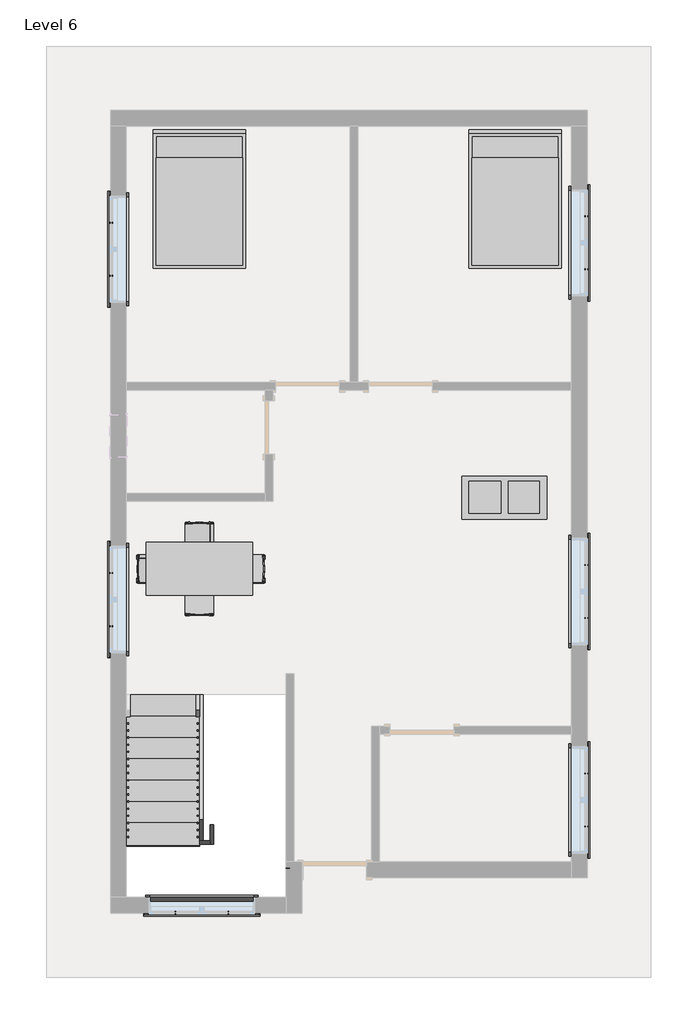
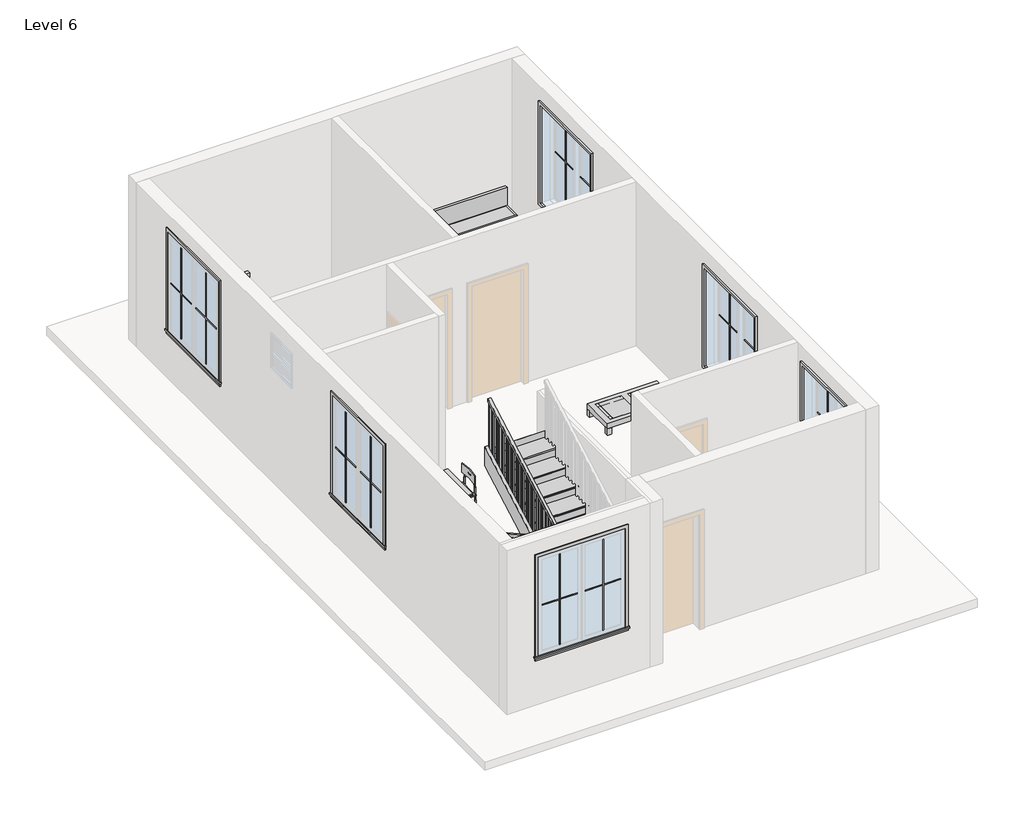
# One storey, part 3 of 3: 25 proxies, 6 members, 3 furniture elements, 1 railing, 1 stair flight.
"""IFC4 building model written with IfcOpenShell, lengths in millimetres."""

from ifc_helpers import new_model, si_unit, frame, origin, place, context, project, spatial, polyline, outline, extrude, faceted_brep, transform, mapped, element, save
from components import muntin_pattern_2x2_muntin_pattern_2x2_f6a80940, muntin_pattern_2x2_muntin_pattern_2x2_09b00a1c, trim_window_exterior_flat_with_sill_698ed857, trim_window_interior_flat_picture_frame_92551a5e, coffee_table_with_brass_mullions_11320_coffee_table_with_5962bef7, bed_17739_bed_17739_15c61121, dining_table_w_chairs_11374_0cdfc61b, stair_flight_f50d1433

model = new_model("IFC4")

# Units and contexts
model_context = context("Model", 3, world=origin())
ifc_project = project(units=[si_unit("LENGTHUNIT", "METRE", prefix="MILLI")], contexts=[model_context])

# Site, building, storey
site = spatial("IfcSite", under=ifc_project)
building = spatial("IfcBuilding", under=site)
storey = spatial("IfcBuildingStorey", under=building, Name="Level 6", Elevation=15849.6)

# Proxies
placement = place(None, origin())
muntin_pattern_2x2_muntin_pattern_2x2_shape = muntin_pattern_2x2_muntin_pattern_2x2_f6a80940(model_context)
element("IfcBuildingElementProxy", 1, Name="Muntin Pattern_2x2 : Muntin Pattern_2x2", ObjectType="Muntin Pattern_2x2 : Muntin Pattern_2x2", at=placement, inside=storey, context=model_context, shape_type="MappedRepresentation", body=[
    mapped(muntin_pattern_2x2_muntin_pattern_2x2_shape, transform((-2773.368364, -6686.2830018, 16833.85), x_axis=(-1.0, 0.0, 0.0), y_axis=(0.0, -1.0, 0.0), z_axis=(0.0, 0.0, 1.0))),
])
element("IfcBuildingElementProxy", 2, Name="Muntin Pattern_2x2 : Muntin Pattern_2x2", ObjectType="Muntin Pattern_2x2 : Muntin Pattern_2x2", at=placement, inside=storey, context=model_context, shape_type="MappedRepresentation", body=[
    mapped(muntin_pattern_2x2_muntin_pattern_2x2_shape, transform((2349.494136, -4693.9705018, 16833.85), x_axis=(0.0, -1.0, 0.0), y_axis=(1.0, 0.0, 0.0), z_axis=(0.0, 0.0, 1.0))),
])
element("IfcBuildingElementProxy", 3, Name="Muntin Pattern_2x2 : Muntin Pattern_2x2", ObjectType="Muntin Pattern_2x2 : Muntin Pattern_2x2", at=placement, inside=storey, context=model_context, shape_type="MappedRepresentation", body=[
    mapped(muntin_pattern_2x2_muntin_pattern_2x2_shape, transform((2349.494136, -1712.6455018, 16833.85), x_axis=(0.0, -1.0, 0.0), y_axis=(1.0, 0.0, 0.0), z_axis=(0.0, 0.0, 1.0))),
])
element("IfcBuildingElementProxy", 4, Name="Muntin Pattern_2x2 : Muntin Pattern_2x2", ObjectType="Muntin Pattern_2x2 : Muntin Pattern_2x2", at=placement, inside=storey, context=model_context, shape_type="MappedRepresentation", body=[
    mapped(muntin_pattern_2x2_muntin_pattern_2x2_shape, transform((-4451.355864, -2586.5525081, 16833.85), x_axis=(0.0, 1.0, 0.0), y_axis=(-1.0, 0.0, 0.0), z_axis=(0.0, 0.0, 1.0))),
])
element("IfcBuildingElementProxy", 5, Name="Muntin Pattern_2x2 : Muntin Pattern_2x2", ObjectType="Muntin Pattern_2x2 : Muntin Pattern_2x2", at=placement, inside=storey, context=model_context, shape_type="MappedRepresentation", body=[
    mapped(muntin_pattern_2x2_muntin_pattern_2x2_shape, transform((2349.494136, 3272.1044982, 16833.85), x_axis=(0.0, -1.0, 0.0), y_axis=(1.0, 0.0, 0.0), z_axis=(0.0, 0.0, 1.0))),
])
element("IfcBuildingElementProxy", 6, Name="Muntin Pattern_2x2 : Muntin Pattern_2x2", ObjectType="Muntin Pattern_2x2 : Muntin Pattern_2x2", at=placement, inside=storey, context=model_context, shape_type="MappedRepresentation", body=[
    mapped(muntin_pattern_2x2_muntin_pattern_2x2_shape, transform((-4451.355864, 2421.2162133, 16833.85), x_axis=(0.0, 1.0, 0.0), y_axis=(-1.0, 0.0, 0.0), z_axis=(0.0, 0.0, 1.0))),
])
muntin_pattern_2x2_muntin_pattern_2x2_2_shape = muntin_pattern_2x2_muntin_pattern_2x2_09b00a1c(model_context)
element("IfcBuildingElementProxy", 7, Name="Muntin Pattern_2x2 : Muntin Pattern_2x2", ObjectType="Muntin Pattern_2x2 : Muntin Pattern_2x2", at=placement, inside=storey, context=model_context, shape_type="MappedRepresentation", body=[
    mapped(muntin_pattern_2x2_muntin_pattern_2x2_2_shape, transform((-3532.193364, -6686.2830018, 16833.85), x_axis=(1.0, 0.0, 0.0), y_axis=(0.0, 1.0, 0.0), z_axis=(0.0, 0.0, 1.0))),
])
element("IfcBuildingElementProxy", 8, Name="Muntin Pattern_2x2 : Muntin Pattern_2x2", ObjectType="Muntin Pattern_2x2 : Muntin Pattern_2x2", at=placement, inside=storey, context=model_context, shape_type="MappedRepresentation", body=[
    mapped(muntin_pattern_2x2_muntin_pattern_2x2_2_shape, transform((2349.494136, -5452.7955018, 16833.85), x_axis=(0.0, 1.0, 0.0), y_axis=(-1.0, 0.0, 0.0), z_axis=(0.0, 0.0, 1.0))),
])
element("IfcBuildingElementProxy", 9, Name="Muntin Pattern_2x2 : Muntin Pattern_2x2", ObjectType="Muntin Pattern_2x2 : Muntin Pattern_2x2", at=placement, inside=storey, context=model_context, shape_type="MappedRepresentation", body=[
    mapped(muntin_pattern_2x2_muntin_pattern_2x2_2_shape, transform((2349.494136, -2471.4705018, 16833.85), x_axis=(0.0, 1.0, 0.0), y_axis=(-1.0, 0.0, 0.0), z_axis=(0.0, 0.0, 1.0))),
])
element("IfcBuildingElementProxy", 10, Name="Muntin Pattern_2x2 : Muntin Pattern_2x2", ObjectType="Muntin Pattern_2x2 : Muntin Pattern_2x2", at=placement, inside=storey, context=model_context, shape_type="MappedRepresentation", body=[
    mapped(muntin_pattern_2x2_muntin_pattern_2x2_2_shape, transform((-4451.355864, -1827.7275081, 16833.85), x_axis=(0.0, -1.0, 0.0), y_axis=(1.0, 0.0, 0.0), z_axis=(0.0, 0.0, 1.0))),
])
element("IfcBuildingElementProxy", 11, Name="Muntin Pattern_2x2 : Muntin Pattern_2x2", ObjectType="Muntin Pattern_2x2 : Muntin Pattern_2x2", at=placement, inside=storey, context=model_context, shape_type="MappedRepresentation", body=[
    mapped(muntin_pattern_2x2_muntin_pattern_2x2_2_shape, transform((2349.494136, 2513.2794982, 16833.85), x_axis=(0.0, 1.0, 0.0), y_axis=(-1.0, 0.0, 0.0), z_axis=(0.0, 0.0, 1.0))),
])
element("IfcBuildingElementProxy", 12, Name="Muntin Pattern_2x2 : Muntin Pattern_2x2", ObjectType="Muntin Pattern_2x2 : Muntin Pattern_2x2", at=placement, inside=storey, context=model_context, shape_type="MappedRepresentation", body=[
    mapped(muntin_pattern_2x2_muntin_pattern_2x2_2_shape, transform((-4451.355864, 3180.0412133, 16833.85), x_axis=(0.0, -1.0, 0.0), y_axis=(1.0, 0.0, 0.0), z_axis=(0.0, 0.0, 1.0))),
])
trim_window_exterior_flat_with_sill_shape = trim_window_exterior_flat_with_sill_698ed857(model_context)
element("IfcBuildingElementProxy", 13, Name="Trim-Window-Exterior-Flat : with Sill", ObjectType="Trim-Window-Exterior-Flat : with Sill", at=placement, inside=storey, context=model_context, shape_type="MappedRepresentation", body=[
    mapped(trim_window_exterior_flat_with_sill_shape, transform((-3152.780864, -6695.8080018, 18592.8), x_axis=(1.0, 0.0, 0.0), y_axis=(0.0, 0.0, 1.0), z_axis=(0.0, -1.0, 0.0))),
])
element("IfcBuildingElementProxy", 14, Name="Trim-Window-Exterior-Flat : with Sill", ObjectType="Trim-Window-Exterior-Flat : with Sill", at=placement, inside=storey, context=model_context, shape_type="MappedRepresentation", body=[
    mapped(trim_window_exterior_flat_with_sill_shape, transform((2359.019136, -5073.3830018, 18592.8), x_axis=(0.0, 1.0, 0.0), y_axis=(0.0, 0.0, 1.0), z_axis=(1.0, 0.0, 0.0))),
])
element("IfcBuildingElementProxy", 15, Name="Trim-Window-Exterior-Flat : with Sill", ObjectType="Trim-Window-Exterior-Flat : with Sill", at=placement, inside=storey, context=model_context, shape_type="MappedRepresentation", body=[
    mapped(trim_window_exterior_flat_with_sill_shape, transform((2359.019136, -2092.0580018, 18592.8), x_axis=(0.0, 1.0, 0.0), y_axis=(0.0, 0.0, 1.0), z_axis=(1.0, 0.0, 0.0))),
])
element("IfcBuildingElementProxy", 16, Name="Trim-Window-Exterior-Flat : with Sill", ObjectType="Trim-Window-Exterior-Flat : with Sill", at=placement, inside=storey, context=model_context, shape_type="MappedRepresentation", body=[
    mapped(trim_window_exterior_flat_with_sill_shape, transform((-4460.880864, -2207.1400081, 18592.8), x_axis=(0.0, -1.0, 0.0), y_axis=(0.0, 0.0, 1.0), z_axis=(-1.0, 0.0, 0.0))),
])
element("IfcBuildingElementProxy", 17, Name="Trim-Window-Exterior-Flat : with Sill", ObjectType="Trim-Window-Exterior-Flat : with Sill", at=placement, inside=storey, context=model_context, shape_type="MappedRepresentation", body=[
    mapped(trim_window_exterior_flat_with_sill_shape, transform((2359.019136, 2892.6919982, 18592.8), x_axis=(0.0, 1.0, 0.0), y_axis=(0.0, 0.0, 1.0), z_axis=(1.0, 0.0, 0.0))),
])
element("IfcBuildingElementProxy", 18, Name="Trim-Window-Exterior-Flat : with Sill", ObjectType="Trim-Window-Exterior-Flat : with Sill", at=placement, inside=storey, context=model_context, shape_type="MappedRepresentation", body=[
    mapped(trim_window_exterior_flat_with_sill_shape, transform((-4460.880864, 2800.6287133, 18592.8), x_axis=(0.0, -1.0, 0.0), y_axis=(0.0, 0.0, 1.0), z_axis=(-1.0, 0.0, 0.0))),
])
trim_window_interior_flat_picture_frame_shape = trim_window_interior_flat_picture_frame_92551a5e(model_context)
element("IfcBuildingElementProxy", 19, Name="Trim-Window-Interior-Flat : Picture Frame", ObjectType="Trim-Window-Interior-Flat : Picture Frame", at=placement, inside=storey, context=model_context, shape_type="MappedRepresentation", body=[
    mapped(trim_window_interior_flat_picture_frame_shape, transform((-3152.780864, -6467.2080018, 18592.8), x_axis=(-1.0, 0.0, 0.0), y_axis=(0.0, 0.0, 1.0), z_axis=(0.0, 1.0, 0.0))),
])
element("IfcBuildingElementProxy", 20, Name="Trim-Window-Interior-Flat : Picture Frame", ObjectType="Trim-Window-Interior-Flat : Picture Frame", at=placement, inside=storey, context=model_context, shape_type="MappedRepresentation", body=[
    mapped(trim_window_interior_flat_picture_frame_shape, transform((2130.419136, -5073.3830018, 18592.8), x_axis=(0.0, -1.0, 0.0), y_axis=(0.0, 0.0, 1.0), z_axis=(-1.0, 0.0, 0.0))),
])
element("IfcBuildingElementProxy", 21, Name="Trim-Window-Interior-Flat : Picture Frame", ObjectType="Trim-Window-Interior-Flat : Picture Frame", at=placement, inside=storey, context=model_context, shape_type="MappedRepresentation", body=[
    mapped(trim_window_interior_flat_picture_frame_shape, transform((2130.419136, -2092.0580018, 18592.8), x_axis=(0.0, -1.0, 0.0), y_axis=(0.0, 0.0, 1.0), z_axis=(-1.0, 0.0, 0.0))),
])
element("IfcBuildingElementProxy", 22, Name="Trim-Window-Interior-Flat : Picture Frame", ObjectType="Trim-Window-Interior-Flat : Picture Frame", at=placement, inside=storey, context=model_context, shape_type="MappedRepresentation", body=[
    mapped(trim_window_interior_flat_picture_frame_shape, transform((-4232.280864, -2207.1400081, 18592.8), x_axis=(0.0, 1.0, 0.0), y_axis=(0.0, 0.0, 1.0), z_axis=(1.0, 0.0, 0.0))),
])
element("IfcBuildingElementProxy", 23, Name="Trim-Window-Interior-Flat : Picture Frame", ObjectType="Trim-Window-Interior-Flat : Picture Frame", at=placement, inside=storey, context=model_context, shape_type="MappedRepresentation", body=[
    mapped(trim_window_interior_flat_picture_frame_shape, transform((2130.419136, 2892.6919982, 18592.8), x_axis=(0.0, -1.0, 0.0), y_axis=(0.0, 0.0, 1.0), z_axis=(-1.0, 0.0, 0.0))),
])
element("IfcBuildingElementProxy", 24, Name="Trim-Window-Interior-Flat : Picture Frame", ObjectType="Trim-Window-Interior-Flat : Picture Frame", at=placement, inside=storey, context=model_context, shape_type="MappedRepresentation", body=[
    mapped(trim_window_interior_flat_picture_frame_shape, transform((-4232.280864, 2800.6287133, 18592.8), x_axis=(0.0, 1.0, 0.0), y_axis=(0.0, 0.0, 1.0), z_axis=(1.0, 0.0, 0.0))),
])
coffee_table_with_brass_mullions_11320_coffee_table_with_shape = coffee_table_with_brass_mullions_11320_coffee_table_with_5962bef7(model_context)
element("IfcBuildingElementProxy", 25, Name="coffee_table_with_brass_mullions_11320 : coffee_table_with_brass_mullions_11320", ObjectType="coffee_table_with_brass_mullions_11320 : coffee_table_with_brass_mullions_11320", at=placement, inside=storey, context=model_context, shape_type="MappedRepresentation", body=[
    mapped(coffee_table_with_brass_mullions_11320_coffee_table_with_shape, transform((1812.3816081, -1181.1001099, 15849.6), x_axis=(1.0, 0.0, 0.0), y_axis=(0.0, 1.0, 0.0), z_axis=(0.0, 0.0, 1.0))),
])

# Furniture
bed_17739_bed_17739_shape = bed_17739_bed_17739_15c61121(model_context)
element("IfcFurniture", 26, ObjectType="Bed_17739 : Bed_17739", at=placement, inside=storey, context=model_context, shape_type="MappedRepresentation", body=[
    mapped(bed_17739_bed_17739_shape, transform((1328.5116081, 3496.3098901, 15849.6), x_axis=(1.0, 0.0, 0.0), y_axis=(0.0, 1.0, 0.0), z_axis=(0.0, 0.0, 1.0))),
])
element("IfcFurniture", 27, ObjectType="Bed_17739 : Bed_17739", at=placement, inside=storey, context=model_context, shape_type="MappedRepresentation", body=[
    mapped(bed_17739_bed_17739_shape, transform((-3187.6083919, 3496.3098901, 15849.6), x_axis=(1.0, 0.0, 0.0), y_axis=(0.0, 1.0, 0.0), z_axis=(0.0, 0.0, 1.0))),
])
dining_table_w_chairs_11374_shape = dining_table_w_chairs_11374_0cdfc61b(model_context)
element("IfcFurniture", 28, ObjectType="Dining_Table_w_Chairs_11374", at=placement, inside=storey, context=model_context, shape_type="MappedRepresentation", body=[
    mapped(dining_table_w_chairs_11374_shape, transform((-3205.8741586, -1863.0511877, 15849.6), x_axis=(1.0, 0.0, 0.0), y_axis=(0.0, 1.0, 0.0), z_axis=(0.0, 0.0, 1.0))),
])

# Members
element("IfcMember", 29, ObjectType="Stringer - 2\" Width", at=placement, inside=storey, context=model_context, shape_type="SweptSolid", body=[
    extrude(outline(polyline([(-3571.6080018, 16057.1983948), (-3571.6080018, 15849.6), (-3825.5525046, 15849.6), (-5654.4080018, 16865.6308318), (-5654.4080018, 17214.3095059), (-3571.6080018, 16057.1983948)])), frame((-3187.6083919, 0.0, 0.0), z_axis=(1.0, 0.0, 0.0), x_axis=(0.0, 1.0, 0.0)), (0.0, 0.0, 1.0), 50.8),
])
element("IfcMember", 30, ObjectType="Stringer - 2\" Width", at=placement, inside=storey, context=model_context, shape_type="SweptSolid", body=[
    extrude(outline(polyline([(-3187.6083919, -5705.2080018), (-3187.6083919, -5654.4080018), (-3035.2083919, -5654.4080018), (-3035.2083919, -5705.2080018), (-3187.6083919, -5705.2080018)])), frame((0.0, 0.0, 16975.6666667), z_axis=(0.0, 0.0, 1.0), x_axis=(1.0, 0.0, 0.0)), (0.0, 0.0, 1.0), 304.8),
])
element("IfcMember", 31, ObjectType="Stringer - 2\" Width", at=placement, inside=storey, context=model_context, shape_type="SweptSolid", body=[
    extrude(outline(polyline([(-5705.2080018, 16975.6666667), (-5705.2080018, 17242.5317281), (-3571.6080018, 18427.8650614), (-3571.6080018, 18079.1863873), (-5557.943499, 16975.6666667), (-5705.2080018, 16975.6666667)])), frame((-3035.2083919, 0.0, 0.0), z_axis=(1.0, 0.0, 0.0), x_axis=(0.0, 1.0, 0.0)), (0.0, 0.0, 1.0), 50.8),
])
element("IfcMember", 32, ObjectType="Stringer - 2\" Width", at=placement, inside=storey, context=model_context, shape_type="SweptSolid", body=[
    extrude(outline(polyline([(-3571.6080018, 16057.1983948), (-3571.6080018, 15849.6), (-3825.5525046, 15849.6), (-6401.1125046, 17280.4666667), (-5773.4908912, 17280.4666667), (-3571.6080018, 16057.1983948)])), frame((-4283.080864, 0.0, 0.0), z_axis=(1.0, 0.0, 0.0), x_axis=(0.0, 1.0, 0.0)), (0.0, 0.0, 1.0), 50.8),
])
element("IfcMember", 33, ObjectType="Stringer - 2\" Width", at=placement, inside=storey, context=model_context, shape_type="SweptSolid", body=[
    extrude(outline(polyline([(-4283.080864, -6518.0080018), (-4283.080864, -6467.2080018), (-1946.280864, -6467.2080018), (-1946.280864, -6518.0080018), (-4283.080864, -6518.0080018)])), frame((0.0, 0.0, 16975.6666667), z_axis=(0.0, 0.0, 1.0), x_axis=(1.0, 0.0, 0.0)), (0.0, 0.0, 1.0), 304.8),
])
element("IfcMember", 34, ObjectType="Stringer - 2\" Width", at=placement, inside=storey, context=model_context, shape_type="SweptSolid", body=[
    extrude(outline(polyline([(-6185.5651124, 16975.6666667), (-3571.6080018, 18427.8650614), (-3571.6080018, 18079.1863873), (-5557.943499, 16975.6666667), (-6185.5651124, 16975.6666667)])), frame((-1946.280864, 0.0, 0.0), z_axis=(1.0, 0.0, 0.0), x_axis=(0.0, 1.0, 0.0)), (0.0, 0.0, 1.0), 50.8),
])

# Railing
element("IfcRailing", 35, ObjectType="Handrail - Rectangular", at=placement, inside=storey, context=model_context, shape_type="SolidModel", body=[
    faceted_brep([(-3187.6083919, -3571.6080018, 16933.3333333), (-3187.6083919, -3571.6080018, 16875.220221), (-3238.4083919, -3571.6080018, 16875.220221), (-3238.4083919, -3571.6080018, 16933.3333333), (-3187.6083919, -5629.0080018, 18076.3333333), (-3187.6083919, -5679.8080018, 18046.4424432), (-3238.4083919, -5679.8080018, 18046.4424432), (-3238.4083919, -5629.0080018, 18076.3333333), (-3187.6083919, -5629.0080018, 18118.6666667), (-3187.6083919, -5679.8080018, 18067.8666667), (-3238.4083919, -5679.8080018, 18067.8666667), (-3238.4083919, -5629.0080018, 18118.6666667), (-3187.6083919, -5705.2080018, 18118.6666667), (-3187.6083919, -5705.2080018, 18067.8666667), (-3238.4083919, -5756.0080018, 18067.8666667), (-3238.4083919, -5756.0080018, 18118.6666667), (-3111.4083919, -5705.2080018, 18118.6666667), (-3111.4083919, -5705.2080018, 18067.8666667), (-3111.4083919, -5756.0080018, 18067.8666667), (-3111.4083919, -5756.0080018, 18118.6666667), (-3060.6083919, -5705.2080018, 18118.6666667), (-3009.8083919, -5705.2080018, 18067.8666667), (-3009.8083919, -5756.0080018, 18067.8666667), (-3060.6083919, -5756.0080018, 18118.6666667), (-3060.6083919, -5705.2080018, 18161.0), (-3009.8083919, -5705.2080018, 18110.2), (-3009.8083919, -5756.0080018, 18110.2), (-3060.6083919, -5756.0080018, 18161.0), (-2984.4083919, -5705.2080018, 18161.0), (-2984.4083919, -5705.2080018, 18110.2), (-2933.6083919, -5756.0080018, 18110.2), (-2933.6083919, -5756.0080018, 18161.0), (-2984.4083919, -5629.0080018, 18161.0), (-2984.4083919, -5615.8443995, 18110.2), (-2933.6083919, -5615.8443995, 18110.2), (-2933.6083919, -5629.0080018, 18161.0), (-2984.4083919, -3571.6080018, 19304.0), (-2933.6083919, -3571.6080018, 19304.0), (-2933.6083919, -3571.6080018, 19245.8868876), (-2984.4083919, -3571.6080018, 19245.8868876)], [[[0, 1, 2, 3]], [[1, 0, 4, 5]], [[2, 1, 5, 6]], [[3, 2, 6, 7]], [[0, 3, 7, 4]], [[5, 4, 8, 9]], [[6, 5, 9, 10]], [[7, 6, 10, 11]], [[4, 7, 11, 8]], [[9, 8, 12, 13]], [[10, 9, 13, 14]], [[11, 10, 14, 15]], [[8, 11, 15, 12]], [[13, 12, 16, 17]], [[14, 13, 17, 18]], [[15, 14, 18, 19]], [[12, 15, 19, 16]], [[17, 16, 20, 21]], [[18, 17, 21, 22]], [[19, 18, 22, 23]], [[16, 19, 23, 20]], [[21, 20, 24, 25]], [[22, 21, 25, 26]], [[23, 22, 26, 27]], [[20, 23, 27, 24]], [[25, 24, 28, 29]], [[26, 25, 29, 30]], [[27, 26, 30, 31]], [[24, 27, 31, 28]], [[29, 28, 32, 33]], [[30, 29, 33, 34]], [[31, 30, 34, 35]], [[28, 31, 35, 32]], [[36, 37, 38, 39]], [[33, 32, 36, 39]], [[34, 33, 39, 38]], [[35, 34, 38, 37]], [[32, 35, 37, 36]]]),
    extrude(outline(polyline([(-3587.4830018, 19237.0674432), (-3587.4830018, 18220.2666667), (-3606.5330018, 18220.2666667), (-3606.5330018, 19226.4841099), (-3587.4830018, 19237.0674432)])), frame((-2968.5333919, 0.0, 0.0), z_axis=(1.0, 0.0, 0.0), x_axis=(0.0, 1.0, 0.0)), (0.0, 0.0, 1.0), 19.05),
    extrude(outline(polyline([(-3689.0830018, 19180.6229988), (-3689.0830018, 18220.2666667), (-3708.1330018, 18220.2666667), (-3708.1330018, 19170.0396654), (-3689.0830018, 19180.6229988)])), frame((-2968.5333919, 0.0, 0.0), z_axis=(1.0, 0.0, 0.0), x_axis=(0.0, 1.0, 0.0)), (0.0, 0.0, 1.0), 19.05),
    extrude(outline(polyline([(-3790.6830018, 19124.1785543), (-3790.6830018, 18220.2666667), (-3809.7330018, 18220.2666667), (-3809.7330018, 19113.595221), (-3790.6830018, 19124.1785543)])), frame((-2968.5333919, 0.0, 0.0), z_axis=(1.0, 0.0, 0.0), x_axis=(0.0, 1.0, 0.0)), (0.0, 0.0, 1.0), 19.05),
    extrude(outline(polyline([(-3892.2830018, 19067.7341099), (-3892.2830018, 18050.9333333), (-3911.3330018, 18050.9333333), (-3911.3330018, 19057.1507765), (-3892.2830018, 19067.7341099)])), frame((-2968.5333919, 0.0, 0.0), z_axis=(1.0, 0.0, 0.0), x_axis=(0.0, 1.0, 0.0)), (0.0, 0.0, 1.0), 19.05),
    extrude(outline(polyline([(-3993.8830018, 19011.2896654), (-3993.8830018, 18050.9333333), (-4012.9330018, 18050.9333333), (-4012.9330018, 19000.7063321), (-3993.8830018, 19011.2896654)])), frame((-2968.5333919, 0.0, 0.0), z_axis=(1.0, 0.0, 0.0), x_axis=(0.0, 1.0, 0.0)), (0.0, 0.0, 1.0), 19.05),
    extrude(outline(polyline([(-4095.4830018, 18954.845221), (-4095.4830018, 18050.9333333), (-4114.5330018, 18050.9333333), (-4114.5330018, 18944.2618876), (-4095.4830018, 18954.845221)])), frame((-2968.5333919, 0.0, 0.0), z_axis=(1.0, 0.0, 0.0), x_axis=(0.0, 1.0, 0.0)), (0.0, 0.0, 1.0), 19.05),
    extrude(outline(polyline([(-4197.0830018, 18898.4007765), (-4197.0830018, 17881.6), (-4216.1330018, 17881.6), (-4216.1330018, 18887.8174432), (-4197.0830018, 18898.4007765)])), frame((-2968.5333919, 0.0, 0.0), z_axis=(1.0, 0.0, 0.0), x_axis=(0.0, 1.0, 0.0)), (0.0, 0.0, 1.0), 19.05),
    extrude(outline(polyline([(-4298.6830018, 18841.9563321), (-4298.6830018, 17881.6), (-4317.7330018, 17881.6), (-4317.7330018, 18831.3729988), (-4298.6830018, 18841.9563321)])), frame((-2968.5333919, 0.0, 0.0), z_axis=(1.0, 0.0, 0.0), x_axis=(0.0, 1.0, 0.0)), (0.0, 0.0, 1.0), 19.05),
    extrude(outline(polyline([(-4400.2830018, 18785.5118876), (-4400.2830018, 17881.6), (-4419.3330018, 17881.6), (-4419.3330018, 18774.9285543), (-4400.2830018, 18785.5118876)])), frame((-2968.5333919, 0.0, 0.0), z_axis=(1.0, 0.0, 0.0), x_axis=(0.0, 1.0, 0.0)), (0.0, 0.0, 1.0), 19.05),
    extrude(outline(polyline([(-4501.8830018, 18729.0674432), (-4501.8830018, 17712.2666667), (-4520.9330018, 17712.2666667), (-4520.9330018, 18718.4841099), (-4501.8830018, 18729.0674432)])), frame((-2968.5333919, 0.0, 0.0), z_axis=(1.0, 0.0, 0.0), x_axis=(0.0, 1.0, 0.0)), (0.0, 0.0, 1.0), 19.05),
    extrude(outline(polyline([(-4603.4830018, 18672.6229988), (-4603.4830018, 17712.2666667), (-4622.5330018, 17712.2666667), (-4622.5330018, 18662.0396654), (-4603.4830018, 18672.6229988)])), frame((-2968.5333919, 0.0, 0.0), z_axis=(1.0, 0.0, 0.0), x_axis=(0.0, 1.0, 0.0)), (0.0, 0.0, 1.0), 19.05),
    extrude(outline(polyline([(-4705.0830018, 18616.1785543), (-4705.0830018, 17712.2666667), (-4724.1330018, 17712.2666667), (-4724.1330018, 18605.595221), (-4705.0830018, 18616.1785543)])), frame((-2968.5333919, 0.0, 0.0), z_axis=(1.0, 0.0, 0.0), x_axis=(0.0, 1.0, 0.0)), (0.0, 0.0, 1.0), 19.05),
    extrude(outline(polyline([(-4806.6830018, 18559.7341099), (-4806.6830018, 17542.9333333), (-4825.7330018, 17542.9333333), (-4825.7330018, 18549.1507765), (-4806.6830018, 18559.7341099)])), frame((-2968.5333919, 0.0, 0.0), z_axis=(1.0, 0.0, 0.0), x_axis=(0.0, 1.0, 0.0)), (0.0, 0.0, 1.0), 19.05),
    extrude(outline(polyline([(-4908.2830018, 18503.2896654), (-4908.2830018, 17542.9333333), (-4927.3330018, 17542.9333333), (-4927.3330018, 18492.7063321), (-4908.2830018, 18503.2896654)])), frame((-2968.5333919, 0.0, 0.0), z_axis=(1.0, 0.0, 0.0), x_axis=(0.0, 1.0, 0.0)), (0.0, 0.0, 1.0), 19.05),
    extrude(outline(polyline([(-5009.8830018, 18446.845221), (-5009.8830018, 17542.9333333), (-5028.9330018, 17542.9333333), (-5028.9330018, 18436.2618876), (-5009.8830018, 18446.845221)])), frame((-2968.5333919, 0.0, 0.0), z_axis=(1.0, 0.0, 0.0), x_axis=(0.0, 1.0, 0.0)), (0.0, 0.0, 1.0), 19.05),
    extrude(outline(polyline([(-5111.4830018, 18390.4007765), (-5111.4830018, 17373.6), (-5130.5330018, 17373.6), (-5130.5330018, 18379.8174432), (-5111.4830018, 18390.4007765)])), frame((-2968.5333919, 0.0, 0.0), z_axis=(1.0, 0.0, 0.0), x_axis=(0.0, 1.0, 0.0)), (0.0, 0.0, 1.0), 19.05),
    extrude(outline(polyline([(-5213.0830018, 18333.9563321), (-5213.0830018, 17373.6), (-5232.1330018, 17373.6), (-5232.1330018, 18323.3729988), (-5213.0830018, 18333.9563321)])), frame((-2968.5333919, 0.0, 0.0), z_axis=(1.0, 0.0, 0.0), x_axis=(0.0, 1.0, 0.0)), (0.0, 0.0, 1.0), 19.05),
    extrude(outline(polyline([(-5314.6830018, 18277.5118876), (-5314.6830018, 17373.6), (-5333.7330018, 17373.6), (-5333.7330018, 18266.9285543), (-5314.6830018, 18277.5118876)])), frame((-2968.5333919, 0.0, 0.0), z_axis=(1.0, 0.0, 0.0), x_axis=(0.0, 1.0, 0.0)), (0.0, 0.0, 1.0), 19.05),
    extrude(outline(polyline([(-5416.2830018, 18221.0674432), (-5416.2830018, 17204.2666667), (-5435.3330018, 17204.2666667), (-5435.3330018, 18210.4841099), (-5416.2830018, 18221.0674432)])), frame((-2968.5333919, 0.0, 0.0), z_axis=(1.0, 0.0, 0.0), x_axis=(0.0, 1.0, 0.0)), (0.0, 0.0, 1.0), 19.05),
    extrude(outline(polyline([(-5517.8830018, 18164.6229988), (-5517.8830018, 17204.2666667), (-5536.9330018, 17204.2666667), (-5536.9330018, 18154.0396654), (-5517.8830018, 18164.6229988)])), frame((-2968.5333919, 0.0, 0.0), z_axis=(1.0, 0.0, 0.0), x_axis=(0.0, 1.0, 0.0)), (0.0, 0.0, 1.0), 19.05),
    extrude(outline(polyline([(-5619.4830018, 18108.1785543), (-5619.4830018, 17204.2666667), (-5638.5330018, 17204.2666667), (-5638.5330018, 18097.595221), (-5619.4830018, 18108.1785543)])), frame((-2968.5333919, 0.0, 0.0), z_axis=(1.0, 0.0, 0.0), x_axis=(0.0, 1.0, 0.0)), (0.0, 0.0, 1.0), 19.05),
    extrude(outline(polyline([(-3019.3333919, -5721.0830018), (-3000.2833919, -5721.0830018), (-3000.2833919, -5740.1330018), (-3019.3333919, -5740.1330018), (-3019.3333919, -5721.0830018)])), frame((0.0, 0.0, 17204.2666667), z_axis=(0.0, 0.0, 1.0), x_axis=(1.0, 0.0, 0.0)), (0.0, 0.0, 1.0), 905.9333333),
    extrude(outline(polyline([(-3120.9333919, -5721.0830018), (-3101.8833919, -5721.0830018), (-3101.8833919, -5740.1330018), (-3120.9333919, -5740.1330018), (-3120.9333919, -5721.0830018)])), frame((0.0, 0.0, 17204.2666667), z_axis=(0.0, 0.0, 1.0), x_axis=(1.0, 0.0, 0.0)), (0.0, 0.0, 1.0), 863.6),
    extrude(outline(polyline([(-3203.4833919, -5695.6830018), (-3203.4833919, -5714.7330018), (-3222.5333919, -5714.7330018), (-3222.5333919, -5695.6830018), (-3203.4833919, -5695.6830018)])), frame((0.0, 0.0, 17204.2666667), z_axis=(0.0, 0.0, 1.0), x_axis=(1.0, 0.0, 0.0)), (0.0, 0.0, 1.0), 863.6),
    extrude(outline(polyline([(-5594.0830018, 17998.8174432), (-5594.0830018, 17034.9333333), (-5613.1330018, 17034.9333333), (-5613.1330018, 18009.4007765), (-5594.0830018, 17998.8174432)])), frame((-3222.5333919, 0.0, 0.0), z_axis=(1.0, 0.0, 0.0), x_axis=(0.0, 1.0, 0.0)), (0.0, 0.0, 1.0), 19.05),
    extrude(outline(polyline([(-5492.4830018, 17942.3729988), (-5492.4830018, 17034.9333333), (-5511.5330018, 17034.9333333), (-5511.5330018, 17952.9563321), (-5492.4830018, 17942.3729988)])), frame((-3222.5333919, 0.0, 0.0), z_axis=(1.0, 0.0, 0.0), x_axis=(0.0, 1.0, 0.0)), (0.0, 0.0, 1.0), 19.05),
    extrude(outline(polyline([(-5390.8830018, 17885.9285543), (-5390.8830018, 17034.9333333), (-5409.9330018, 17034.9333333), (-5409.9330018, 17896.5118876), (-5390.8830018, 17885.9285543)])), frame((-3222.5333919, 0.0, 0.0), z_axis=(1.0, 0.0, 0.0), x_axis=(0.0, 1.0, 0.0)), (0.0, 0.0, 1.0), 19.05),
    extrude(outline(polyline([(-5289.2830018, 17829.4841099), (-5289.2830018, 16865.6), (-5308.3330018, 16865.6), (-5308.3330018, 17840.0674432), (-5289.2830018, 17829.4841099)])), frame((-3222.5333919, 0.0, 0.0), z_axis=(1.0, 0.0, 0.0), x_axis=(0.0, 1.0, 0.0)), (0.0, 0.0, 1.0), 19.05),
    extrude(outline(polyline([(-5187.6830018, 17773.0396654), (-5187.6830018, 16865.6), (-5206.7330018, 16865.6), (-5206.7330018, 17783.6229988), (-5187.6830018, 17773.0396654)])), frame((-3222.5333919, 0.0, 0.0), z_axis=(1.0, 0.0, 0.0), x_axis=(0.0, 1.0, 0.0)), (0.0, 0.0, 1.0), 19.05),
    extrude(outline(polyline([(-5086.0830018, 17716.595221), (-5086.0830018, 16865.6), (-5105.1330018, 16865.6), (-5105.1330018, 17727.1785543), (-5086.0830018, 17716.595221)])), frame((-3222.5333919, 0.0, 0.0), z_axis=(1.0, 0.0, 0.0), x_axis=(0.0, 1.0, 0.0)), (0.0, 0.0, 1.0), 19.05),
    extrude(outline(polyline([(-4984.4830018, 17660.1507765), (-4984.4830018, 16696.2666667), (-5003.5330018, 16696.2666667), (-5003.5330018, 17670.7341099), (-4984.4830018, 17660.1507765)])), frame((-3222.5333919, 0.0, 0.0), z_axis=(1.0, 0.0, 0.0), x_axis=(0.0, 1.0, 0.0)), (0.0, 0.0, 1.0), 19.05),
    extrude(outline(polyline([(-4882.8830018, 17603.7063321), (-4882.8830018, 16696.2666667), (-4901.9330018, 16696.2666667), (-4901.9330018, 17614.2896654), (-4882.8830018, 17603.7063321)])), frame((-3222.5333919, 0.0, 0.0), z_axis=(1.0, 0.0, 0.0), x_axis=(0.0, 1.0, 0.0)), (0.0, 0.0, 1.0), 19.05),
    extrude(outline(polyline([(-4781.2830018, 17547.2618876), (-4781.2830018, 16696.2666667), (-4800.3330018, 16696.2666667), (-4800.3330018, 17557.845221), (-4781.2830018, 17547.2618876)])), frame((-3222.5333919, 0.0, 0.0), z_axis=(1.0, 0.0, 0.0), x_axis=(0.0, 1.0, 0.0)), (0.0, 0.0, 1.0), 19.05),
    extrude(outline(polyline([(-4679.6830018, 17490.8174432), (-4679.6830018, 16526.9333333), (-4698.7330018, 16526.9333333), (-4698.7330018, 17501.4007765), (-4679.6830018, 17490.8174432)])), frame((-3222.5333919, 0.0, 0.0), z_axis=(1.0, 0.0, 0.0), x_axis=(0.0, 1.0, 0.0)), (0.0, 0.0, 1.0), 19.05),
    extrude(outline(polyline([(-4578.0830018, 17434.3729988), (-4578.0830018, 16526.9333333), (-4597.1330018, 16526.9333333), (-4597.1330018, 17444.9563321), (-4578.0830018, 17434.3729988)])), frame((-3222.5333919, 0.0, 0.0), z_axis=(1.0, 0.0, 0.0), x_axis=(0.0, 1.0, 0.0)), (0.0, 0.0, 1.0), 19.05),
    extrude(outline(polyline([(-4476.4830018, 17377.9285543), (-4476.4830018, 16526.9333333), (-4495.5330018, 16526.9333333), (-4495.5330018, 17388.5118876), (-4476.4830018, 17377.9285543)])), frame((-3222.5333919, 0.0, 0.0), z_axis=(1.0, 0.0, 0.0), x_axis=(0.0, 1.0, 0.0)), (0.0, 0.0, 1.0), 19.05),
    extrude(outline(polyline([(-4374.8830018, 17321.4841099), (-4374.8830018, 16357.6), (-4393.9330018, 16357.6), (-4393.9330018, 17332.0674432), (-4374.8830018, 17321.4841099)])), frame((-3222.5333919, 0.0, 0.0), z_axis=(1.0, 0.0, 0.0), x_axis=(0.0, 1.0, 0.0)), (0.0, 0.0, 1.0), 19.05),
    extrude(outline(polyline([(-4273.2830018, 17265.0396654), (-4273.2830018, 16357.6), (-4292.3330018, 16357.6), (-4292.3330018, 17275.6229988), (-4273.2830018, 17265.0396654)])), frame((-3222.5333919, 0.0, 0.0), z_axis=(1.0, 0.0, 0.0), x_axis=(0.0, 1.0, 0.0)), (0.0, 0.0, 1.0), 19.05),
    extrude(outline(polyline([(-4171.6830018, 17208.595221), (-4171.6830018, 16357.6), (-4190.7330018, 16357.6), (-4190.7330018, 17219.1785543), (-4171.6830018, 17208.595221)])), frame((-3222.5333919, 0.0, 0.0), z_axis=(1.0, 0.0, 0.0), x_axis=(0.0, 1.0, 0.0)), (0.0, 0.0, 1.0), 19.05),
    extrude(outline(polyline([(-4070.0830018, 17152.1507765), (-4070.0830018, 16188.2666667), (-4089.1330018, 16188.2666667), (-4089.1330018, 17162.7341099), (-4070.0830018, 17152.1507765)])), frame((-3222.5333919, 0.0, 0.0), z_axis=(1.0, 0.0, 0.0), x_axis=(0.0, 1.0, 0.0)), (0.0, 0.0, 1.0), 19.05),
    extrude(outline(polyline([(-3968.4830018, 17095.7063321), (-3968.4830018, 16188.2666667), (-3987.5330018, 16188.2666667), (-3987.5330018, 17106.2896654), (-3968.4830018, 17095.7063321)])), frame((-3222.5333919, 0.0, 0.0), z_axis=(1.0, 0.0, 0.0), x_axis=(0.0, 1.0, 0.0)), (0.0, 0.0, 1.0), 19.05),
    extrude(outline(polyline([(-3866.8830018, 17039.2618876), (-3866.8830018, 16188.2666667), (-3885.9330018, 16188.2666667), (-3885.9330018, 17049.845221), (-3866.8830018, 17039.2618876)])), frame((-3222.5333919, 0.0, 0.0), z_axis=(1.0, 0.0, 0.0), x_axis=(0.0, 1.0, 0.0)), (0.0, 0.0, 1.0), 19.05),
    extrude(outline(polyline([(-3765.2830018, 16982.8174432), (-3765.2830018, 16018.9333333), (-3784.3330018, 16018.9333333), (-3784.3330018, 16993.4007765), (-3765.2830018, 16982.8174432)])), frame((-3222.5333919, 0.0, 0.0), z_axis=(1.0, 0.0, 0.0), x_axis=(0.0, 1.0, 0.0)), (0.0, 0.0, 1.0), 19.05),
    extrude(outline(polyline([(-3663.6830018, 16926.3729988), (-3663.6830018, 16018.9333333), (-3682.7330018, 16018.9333333), (-3682.7330018, 16936.9563321), (-3663.6830018, 16926.3729988)])), frame((-3222.5333919, 0.0, 0.0), z_axis=(1.0, 0.0, 0.0), x_axis=(0.0, 1.0, 0.0)), (0.0, 0.0, 1.0), 19.05),
    extrude(outline(polyline([(-2968.5333919, -5721.0830018), (-2949.4833919, -5721.0830018), (-2949.4833919, -5740.1330018), (-2968.5333919, -5740.1330018), (-2968.5333919, -5721.0830018)])), frame((0.0, 0.0, 17204.2666667), z_axis=(0.0, 0.0, 1.0), x_axis=(1.0, 0.0, 0.0)), (0.0, 0.0, 1.0), 905.9333333),
    extrude(outline(polyline([(-3203.4833919, -5721.0830018), (-3203.4833919, -5740.1330018), (-3222.5333919, -5740.1330018), (-3222.5333919, -5721.0830018), (-3203.4833919, -5721.0830018)])), frame((0.0, 0.0, 17204.2666667), z_axis=(0.0, 0.0, 1.0), x_axis=(1.0, 0.0, 0.0)), (0.0, 0.0, 1.0), 863.6),
    extrude(outline(polyline([(-3571.6080018, 19245.8868876), (-3571.6080018, 18220.2666667), (-3590.6580018, 18220.2666667), (-3590.6580018, 19235.3035543), (-3571.6080018, 19245.8868876)])), frame((-2968.5333919, 0.0, 0.0), z_axis=(1.0, 0.0, 0.0), x_axis=(0.0, 1.0, 0.0)), (0.0, 0.0, 1.0), 19.05),
    extrude(outline(polyline([(-3571.6080018, 16875.220221), (-3571.6080018, 16018.9333333), (-3590.6580018, 16018.9333333), (-3590.6580018, 16885.8035543), (-3571.6080018, 16875.220221)])), frame((-3222.5333919, 0.0, 0.0), z_axis=(1.0, 0.0, 0.0), x_axis=(0.0, 1.0, 0.0)), (0.0, 0.0, 1.0), 19.05),
])

# Stair flight
stair_flight_shape = stair_flight_f50d1433(model_context)
element("IfcStairFlight", 36, ObjectType="2\" Tread 1\" Nosing 1/4\" Riser", at=placement, inside=storey, context=model_context, shape_type="MappedRepresentation", body=[
    mapped(stair_flight_shape, transform((0.0, 0.0, 0.0), x_axis=(1.0, 0.0, 0.0), y_axis=(0.0, 1.0, 0.0), z_axis=(0.0, 0.0, 1.0))),
])

save(model, "model.ifc")

# Revit data of these elements
# Type "Muntin Pattern_2x2 : Muntin Pattern_2x2"
#   Width [instance default] = 4' - 0"
#   Thickness = 0' - 0 1/2"
#   Height [instance default] = 4' - 0"
#   Distance = 0' - 0 3/4"
#   Interior Material [instance default] = none
#   Exterior Material [instance default] = none
#   Default Elevation = 0
# Type "Trim-Window-Exterior-Flat : with Sill"
#   Trim Width = 0' - 2 1/4"
#   Trim Thickness_Picture Frame = 0' - 1 1/4"
#   Trim Thickness_with Sill = 0' - 0 3/4"
#   Sill Thickness = 0' - 1 1/4"
#   Opening Width [instance default] = 2' - 0"
#   Opening Height [instance default] = 3' - 0"
#   Default Elevation = 4' - 0"
#   Sill = yes
#   Picture Frame = no
#   Trim Material [instance default] = none
# Type "Trim-Window-Interior-Flat : Picture Frame"
#   Trim Thickness_Picture Frame = 0' - 1 1/4"
#   Trim Width = 0' - 2 1/4"
#   Trim Thickness_with Sill = 0' - 0 3/4"
#   Sill Thickness = 0' - 1 1/4"
#   Opening Width [instance default] = 2' - 0"
#   Opening Height [instance default] = 3' - 0"
#   Default Elevation = 4' - 0"
#   Sill = no
#   Picture Frame = yes
#   Trim Material [instance default] = none
# Type "coffee_table_with_brass_mullions_11320 : coffee_table_with_brass_mullions_11320"
#   Default Elevation = 0
# Type "Bed_17739 : Bed_17739"
#   Default Elevation = 0
# Type "Dining_Table_w_Chairs_11374"
#   Default Elevation = 0
#   Assembly Code = ""
# Type "Handrail - Rectangular"
#   Assembly Code = "C2010400"
#   built-in parameter 1008612 = 0.0416667 (stored number, unit not read)
#   built-in parameter 1008611 = 0.0416667 (stored number, unit not read)
#   built-in parameter 1008609 = 0.333333 (stored number, unit not read)
#   built-in parameter 1008604 = 0.166667 (stored number, unit not read)
#   built-in parameter 1008603 = 0.166667 (stored number, unit not read)
#   Railing Height = 3' - 0"
#   built-in parameter 1008630 = 2
#   built-in parameter 1008610 = 2
#   built-in parameter 1008618 = Baluster - Square : 3/4"
# Elements 1, 2, 3, 4, 5, 6, 7, 8, 9, 10, 11, 12 (IfcBuildingElementProxy, "Muntin Pattern_2x2 : Muntin Pattern_2x2")
#   Width = 2' - 0 5/8"
#   Height = 5' - 6 1/2"
#   Interior Material = Wood - Stained
#   Exterior Material = Clad - White
#   Phase Created = New Construction
#   Materials on its faces: "Clad - White", "Wood - Stained"
# Elements 13, 14, 15, 16, 17, 18 (IfcBuildingElementProxy, "Trim-Window-Exterior-Flat : with Sill")
#   Opening Width = 5' - 0"
#   Opening Height = 6' - 0"
#   Trim Material = Clad - White
#   Phase Created = New Construction
#   Materials on its faces: "Clad - White"
# Elements 19, 20, 21, 22, 23, 24 (IfcBuildingElementProxy, "Trim-Window-Interior-Flat : Picture Frame")
#   Opening Width = 5' - 0"
#   Opening Height = 6' - 0"
#   Trim Material = Wood - Stained
#   Phase Created = New Construction
#   Materials on its faces: "Wood - Stained"
# Element 25 (IfcBuildingElementProxy, "coffee_table_with_brass_mullions_11320 : coffee_table_with_brass_mullions_11320")
#   Phase Created = New Construction
#   Materials on its faces: "Default Wall", "TABLE", "Glass", "Default"
# Elements 26, 27 (IfcFurniture, "Bed_17739 : Bed_17739")
#   Phase Created = New Construction
#   Materials on its faces: "legs", "sheets", "bed frame", "Blanket"
# Element 28 (IfcFurniture, "Dining_Table_w_Chairs_11374")
#   Phase Created = New Construction
# Elements 29, 30, 31, 32, 33, 34 (IfcMember, "Stringer - 2\" Width")
#   Phase Created = New Construction
# Element 35 (IfcRailing, "Handrail - Rectangular")
#   Phase Created = New Construction
# Element 36 (IfcStairFlight, "2\" Tread 1\" Nosing 1/4\" Riser")
#   Phase Created = New Construction
# Materials
#   "Clad - White": class "Wood", colour RGB 242 242 238, transparency 0, Cost = 0
#   "Wood - Stained": class "Wood", colour RGB 224 178 126, transparency 0, Cost = 0
#   "Default Wall": colour RGB 128 128 128, transparency 0, Cost = 0
#   "TABLE": class "Generic", colour RGB 120 120 120, transparency 0, Cost = 0
#   "Glass": class "Glass", colour RGB 0 128 192, transparency 0.75, Description = "Soda Lime Glass", Cost = 0
#   "Default": colour RGB 127 127 127, transparency 0, Cost = 0
#   "legs": colour RGB 90 73 37, transparency 0, Cost = 0
#   "sheets": colour RGB 200 195 176, transparency 0, Cost = 0
#   "bed frame": colour RGB 90 73 37, transparency 0, Cost = 0
#   "Blanket": class "System", colour RGB 59 0 1, transparency 0, Cost = 0
